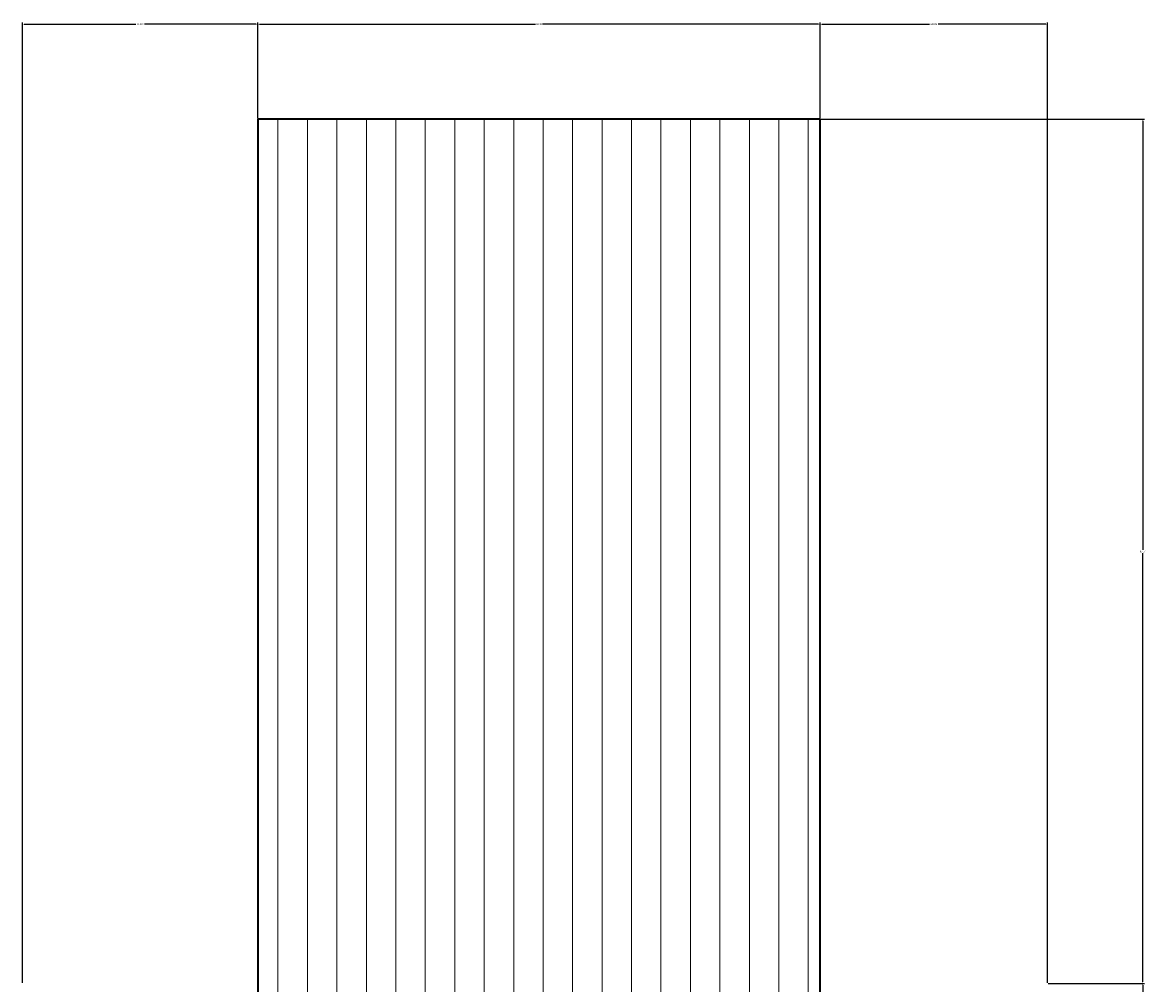
# Model space of a CAD drawing. Units: millimetres. Extents: x 446512 to 447461, y 70395 to 70610.
# Tile 39 of 39: x 447340 to 447461, y 70507 to 70610. Entities that reach past the tile are written whole.
import ezdxf

# ---------------------------------------------------------------- set-up
doc = ezdxf.new("R2010")
doc.units = ezdxf.units.MM
for name, color, linetype, lineweight in [('A-ANNO-DIMS', 2, 'Continuous', 18), ('A-FURN', 7, 'Continuous', 35), ('A-FURN-PATT', 38, 'Continuous', 13)]:
    doc.layers.add(name, color=color, linetype=linetype, lineweight=lineweight)
doc.styles.get("Standard").update_dxf_attribs({"font": 'arial.ttf'})
doc.dimstyles.get("Standard").update_dxf_attribs({"dimtxt": 0.18, "dimasz": 0.18, "dimexe": 0.18, "dimexo": 0.0625, "dimgap": 0.09, "dimtad": 0, "dimtih": 1, "dimtoh": 1, "dimdec": 4, "dimzin": 0, "dimdsep": 46, "dimtxsty": 'Standard', "dimcen": 0.09, "dimadec": 0, "dimazin": 0, "dimtfac": 1, "dimtdec": 4, "dimtofl": 0, "dimtmove": 0, "dimatfit": 3, "dimfxl": 1, "dimtolj": 1, "dimtzin": 0, "dimarcsym": 0})

# ---------------------------------------------------------------- blocks, each defined once
blk = doc.blocks.new('*D64')
at = {"layer": 'A-ANNO-DIMS', "color": 0, "lineweight": -2, "transparency": 16777216}
for p, q in [((447340.05, 70506.61), (447340.05, 70610.14)), ((447340.23, 70609.96), (447352.27, 70609.96)), ((447365.25, 70609.96), (447353.2, 70609.96)), ((447365.43, 70599.78), (447365.43, 70610.14))]:
    blk.add_line(p, q, dxfattribs=at)
at = {"layer": 'A-ANNO-DIMS', "color": 0, "transparency": 16777216}
for points in [[(447340.23, 70609.99), (447340.23, 70609.93), (447340.05, 70609.96)], [(447365.25, 70609.99), (447365.25, 70609.93), (447365.43, 70609.96)]]:
    blk.add_solid(points, dxfattribs=at)
at = {"layer": 'Defpoints', "color": 0, "transparency": 16777216}
for p in [(447365.43, 70609.96), (447365.43, 70599.71), (447340.05, 70506.55)]:
    blk.add_point(p, dxfattribs=at)
at = {"layer": 'A-ANNO-DIMS', "color": 0, "transparency": 16777216, "insert": (447352.74, 70609.96), "char_height": 0.18, "attachment_point": 5}
blk.add_mtext('\\A1;25.376', dxfattribs=at)
blk = doc.blocks.new('*D65')
at = {"layer": 'A-ANNO-DIMS', "color": 0, "lineweight": -2, "transparency": 16777216}
for p, q in [((447365.43, 70599.78), (447365.43, 70610.14)), ((447365.61, 70609.96), (447395.33, 70609.96)), ((447425.83, 70609.96), (447396.11, 70609.96)), ((447426.01, 70599.78), (447426.01, 70610.14))]:
    blk.add_line(p, q, dxfattribs=at)
at = {"layer": 'A-ANNO-DIMS', "color": 0, "transparency": 16777216}
for points in [[(447365.61, 70609.99), (447365.61, 70609.93), (447365.43, 70609.96)], [(447425.83, 70609.99), (447425.83, 70609.93), (447426.01, 70609.96)]]:
    blk.add_solid(points, dxfattribs=at)
at = {"layer": 'Defpoints', "color": 0, "transparency": 16777216}
for p in [(447426.01, 70609.96), (447365.43, 70599.71), (447426.01, 70599.71)]:
    blk.add_point(p, dxfattribs=at)
at = {"layer": 'A-ANNO-DIMS', "color": 0, "transparency": 16777216, "insert": (447395.72, 70609.96), "char_height": 0.18, "attachment_point": 5}
blk.add_mtext('\\A1;60.59', dxfattribs=at)
blk = doc.blocks.new('*D66')
at = {"layer": 'A-ANNO-DIMS', "color": 0, "lineweight": -2, "transparency": 16777216}
for p, q in [((447426.01, 70599.78), (447426.01, 70610.14)), ((447426.19, 70609.96), (447437.81, 70609.96)), ((447450.35, 70609.96), (447438.74, 70609.96)), ((447450.53, 70506.61), (447450.53, 70610.14))]:
    blk.add_line(p, q, dxfattribs=at)
at = {"layer": 'A-ANNO-DIMS', "color": 0, "transparency": 16777216}
for points in [[(447426.19, 70609.99), (447426.19, 70609.93), (447426.01, 70609.96)], [(447450.35, 70609.99), (447450.35, 70609.93), (447450.53, 70609.96)]]:
    blk.add_solid(points, dxfattribs=at)
at = {"layer": 'Defpoints', "color": 0, "transparency": 16777216}
for p in [(447450.53, 70609.96), (447426.01, 70599.71), (447450.53, 70506.55)]:
    blk.add_point(p, dxfattribs=at)
at = {"layer": 'A-ANNO-DIMS', "color": 0, "transparency": 16777216, "insert": (447438.27, 70609.96), "char_height": 0.18, "attachment_point": 5}
blk.add_mtext('\\A1;24.518', dxfattribs=at)
blk = doc.blocks.new('*D70')
at = {"layer": 'A-ANNO-DIMS', "color": 0, "lineweight": -2, "transparency": 16777216}
for p, q in [((447450.59, 70506.55), (447460.96, 70506.55)), ((447460.78, 70506.37), (447460.78, 70504.71)), ((447460.78, 70502.69), (447460.78, 70504.35)), ((447450.59, 70502.51), (447460.96, 70502.51))]:
    blk.add_line(p, q, dxfattribs=at)
at = {"layer": 'A-ANNO-DIMS', "color": 0, "transparency": 16777216}
for points in [[(447460.75, 70506.37), (447460.81, 70506.37), (447460.78, 70506.55)], [(447460.75, 70502.69), (447460.81, 70502.69), (447460.78, 70502.51)]]:
    blk.add_solid(points, dxfattribs=at)
at = {"layer": 'Defpoints', "color": 0, "transparency": 16777216}
for p in [(447450.53, 70506.55), (447460.78, 70506.55), (447450.53, 70502.51)]:
    blk.add_point(p, dxfattribs=at)
at = {"layer": 'A-ANNO-DIMS', "color": 0, "transparency": 16777216, "insert": (447460.78, 70504.53), "char_height": 0.18, "attachment_point": 5}
blk.add_mtext('\\A1;4.035', dxfattribs=at)
blk = doc.blocks.new('*D71')
at = {"layer": 'A-ANNO-DIMS', "color": 0, "lineweight": -2, "transparency": 16777216}
for p, q in [((447426.08, 70599.71), (447460.96, 70599.71)), ((447460.78, 70599.53), (447460.78, 70553.31)), ((447460.78, 70506.73), (447460.78, 70552.95)), ((447450.59, 70506.55), (447460.96, 70506.55))]:
    blk.add_line(p, q, dxfattribs=at)
at = {"layer": 'A-ANNO-DIMS', "color": 0, "transparency": 16777216}
for points in [[(447460.75, 70599.53), (447460.81, 70599.53), (447460.78, 70599.71)], [(447460.75, 70506.73), (447460.81, 70506.73), (447460.78, 70506.55)]]:
    blk.add_solid(points, dxfattribs=at)
at = {"layer": 'Defpoints', "color": 0, "transparency": 16777216}
for p in [(447426.01, 70599.71), (447460.78, 70599.71), (447450.53, 70506.55)]:
    blk.add_point(p, dxfattribs=at)
at = {"layer": 'A-ANNO-DIMS', "color": 0, "transparency": 16777216, "insert": (447460.78, 70553.13), "char_height": 0.18, "attachment_point": 5}
blk.add_mtext('\\A1;93.17', dxfattribs=at)

msp = doc.modelspace()

# ---------------------------------------------------------------- hatches: boundary and pattern name
at = {"layer": 'A-FURN-PATT'}
h = msp.add_hatch(dxfattribs=at)
h.set_pattern_fill('ANSI31', color=256, angle=45)
h.set_pattern_definition([(90, (127.5626, 0), (-3.175, 0), [])])
h.paths.add_polyline_path([(447426.0142, 70599.7147), (447365.4251, 70599.7147), (447365.4251, 70405.3145), (447426.0142, 70405.3145)])

# ---------------------------------------------------------------- linework, layer by layer
at = {"layer": 'A-FURN'}
for p, q in [((447426.0142, 70599.7147), (447365.4251, 70599.7147)), ((447365.4251, 70599.7147), (447365.4251, 70405.3145)), ((447426.0142, 70405.3145), (447426.0142, 70599.7147))]:
    msp.add_line(p, q, dxfattribs=at)

# ---------------------------------------------------------------- dimensions: what is measured, and where the dimension line sits
at = {"layer": 'A-ANNO-DIMS'}
for base, p1, p2, override, picture, middle in [((447365.4251, 70609.9647), (447340.0494, 70506.5496), (447365.4251, 70599.7147), {"dimdec": 3, "dimlfac": 1, "dimrnd": 0, "dimzin": 0, "dimdsep": 46, "dimlunit": 2}, '*D64', (447352.7372, 70609.9647)), ((447426.0142, 70609.9647), (447365.4251, 70599.7147), (447426.0142, 70599.7147), {"dimdec": 2, "dimlfac": 1, "dimrnd": 0, "dimzin": 0, "dimdsep": 46, "dimlunit": 2}, '*D65', (447395.7196, 70609.9647)), ((447450.5318, 70609.9647), (447426.0142, 70599.7147), (447450.5318, 70506.5496), {"dimdec": 3, "dimlfac": 1, "dimrnd": 0, "dimzin": 0, "dimdsep": 46, "dimlunit": 2}, '*D66', (447438.273, 70609.9647))]:
    dim = msp.add_linear_dim(base=base, p1=p1, p2=p2, dimstyle='Standard', override=override, dxfattribs=at)
    dim.commit()
    dim.dimension.update_dxf_attribs({"geometry": picture, "text_midpoint": middle})
for base, p1, p2, override, picture, middle in [((447460.7818, 70599.7147), (447450.5318, 70506.5496), (447426.0142, 70599.7147), {"dimdec": 2, "dimlfac": 1, "dimrnd": 0, "dimzin": 0, "dimdsep": 46, "dimlunit": 2}, '*D71', (447460.7818, 70553.1321)), ((447460.7818, 70506.5496), (447450.5318, 70502.5146), (447450.5318, 70506.5496), {"dimdec": 3, "dimlfac": 1, "dimrnd": 0, "dimzin": 0, "dimdsep": 46, "dimlunit": 2}, '*D70', (447460.7818, 70504.5321))]:
    dim = msp.add_linear_dim(base=base, p1=p1, p2=p2, angle=90, dimstyle='Standard', override=override, dxfattribs=at)
    dim.commit()
    dim.dimension.update_dxf_attribs({"geometry": picture, "text_midpoint": middle})

doc.saveas('drawing.dxf')
